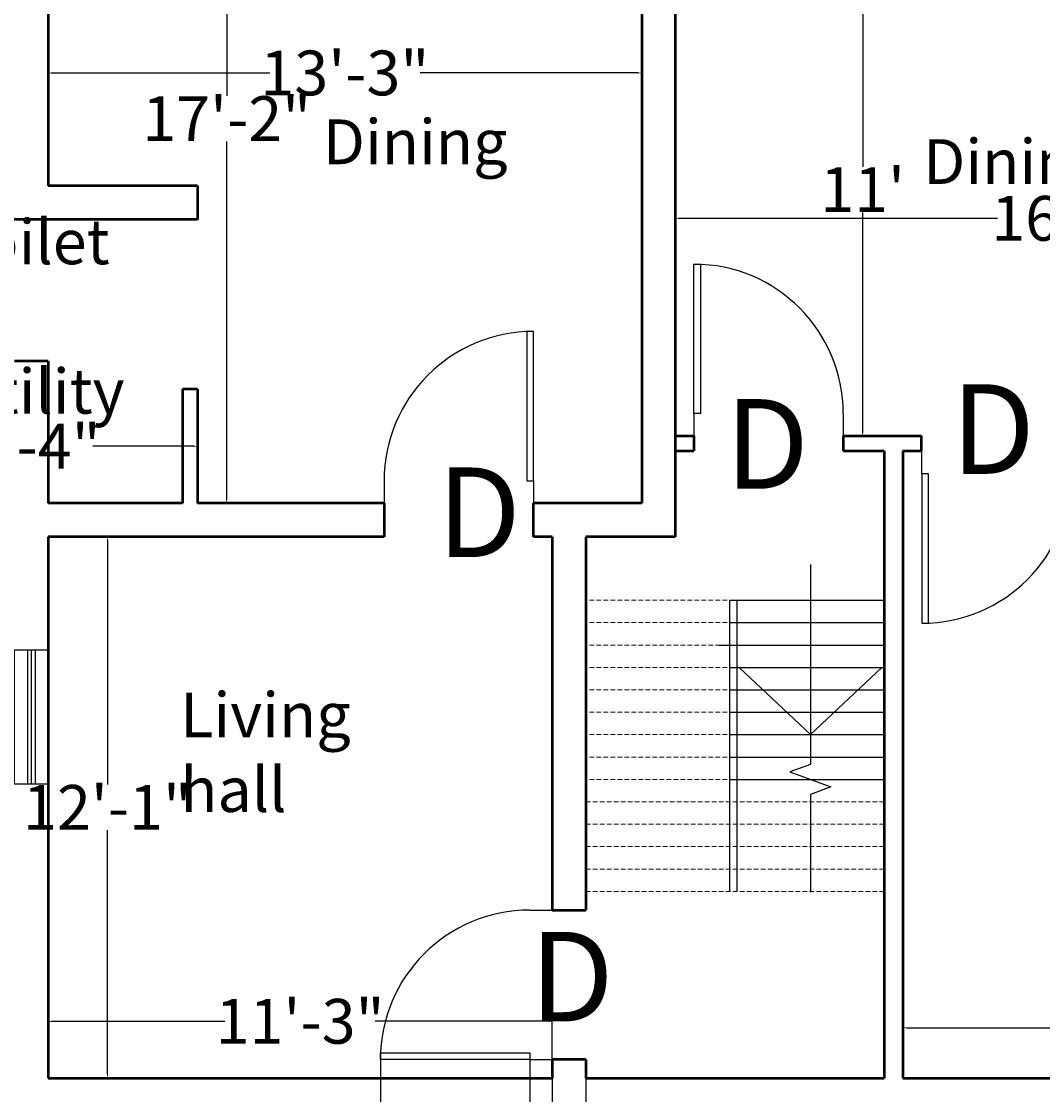
# Model space of a CAD drawing. Units: inches. Extents: x 409 to 7572, y 7 to 725.
# Tile 9 of 38: x 1698 to 1972, y 161 to 449. Entities that reach past the tile are written whole.
import ezdxf

# ---------------------------------------------------------------- set-up
doc = ezdxf.new("R2010")
doc.units = ezdxf.units.IN
doc.header["$MEASUREMENT"] = 0
doc.linetypes.add('HIDDEN', pattern=[0.375, 0.25, -0.125])
for name, color, linetype, lineweight in [('A-ANNO-DIMS', 2, 'Continuous', 18), ('A-ANNO-SYMB', 3, 'Continuous', 25), ('A-AREA-IDEN', 7, 'Continuous', 25), ('A-DOOR', 3, 'Continuous', 25), ('A-FLOR-STRS', 6, 'Continuous', 25), ('A-FLOR-STRS-OVHD', 6, 'HIDDEN', 18), ('A-GLAZ', 4, 'Continuous', 25), ('A-WALL', 7, 'Continuous', 50)]:
    doc.layers.add(name, color=color, linetype=linetype, lineweight=lineweight)
doc.styles.get("Standard").update_dxf_attribs({"font": 'arial.ttf'})
doc.dimstyles.get("Standard").update_dxf_attribs({"dimtxt": 2, "dimasz": 1, "dimexe": 0.18, "dimexo": 0.0625, "dimgap": 0.09, "dimtad": 0, "dimtih": 1, "dimtoh": 1, "dimdec": 0, "dimzin": 0, "dimdsep": 46, "dimlunit": 3, "dimtxsty": 'Standard', "dimcen": 0.09, "dimadec": 0, "dimazin": 0, "dimtfac": 1, "dimtdec": 0, "dimtofl": 0, "dimtmove": 0, "dimatfit": 3, "dimfxl": 1, "dimtolj": 1, "dimtzin": 0, "dimarcsym": 0})

# ---------------------------------------------------------------- blocks, each defined once
blk = doc.blocks.new('*U2')
for p, q in [((0, 0), (0, -6)), ((-40, 0), (-40, -6))]:
    blk.add_line(p, q)
blk.add_lwpolyline([(0, 0), (0, 40), (-1.75, 40), (-1.75, 0)], close=True)
blk.add_arc((0, 0), 40, 90, 180)
blk = doc.blocks.new('*U3')
for p, q in [((0, 0), (0, -6)), ((40, 0), (40, -6))]:
    blk.add_line(p, q)
blk.add_lwpolyline([(0, 0), (0, 40), (1.75, 40), (1.75, 0)], close=True)
blk.add_arc((0, 0), 40, 0, 90)
blk = doc.blocks.new('*U4')
for p, q in [((0, 0), (0, -6)), ((40, 0), (40, -6))]:
    blk.add_line(p, q)
blk.add_lwpolyline([(0, 0), (0, 40), (1.75, 40), (1.75, 0)], close=True)
blk.add_arc((0, 0), 40, 0, 90)
blk = doc.blocks.new('*U5')
for p, q in [((0, 0), (0, 6)), ((40, 0), (40, 6))]:
    blk.add_line(p, q)
blk.add_lwpolyline([(0, 0), (0, -40), (1.75, -40), (1.75, 0)], close=True)
blk.add_arc((0, 0), 40, 270, 0)
blk = doc.blocks.new('*D40')
at = {"layer": 'A-ANNO-DIMS', "color": 0, "lineweight": -2, "transparency": 16777216}
for p, q in [((1934.32, 165.59), (1934.32, 179.18)), ((1935.32, 179), (1982.18, 179)), ((2069.32, 179), (2022.46, 179)), ((2070.32, 165.59), (2070.32, 179.18))]:
    blk.add_line(p, q, dxfattribs=at)
at = {"layer": 'A-ANNO-DIMS', "color": 0, "transparency": 16777216}
for points in [[(1935.32, 179.16), (1935.32, 178.83), (1934.32, 179)], [(2069.32, 179.16), (2069.32, 178.83), (2070.32, 179)]]:
    blk.add_solid(points, dxfattribs=at)
at = {"layer": 'DEFPOINTS', "color": 0, "transparency": 16777216}
for p in [(2070.32, 179), (1934.32, 165.53), (2070.32, 165.53)]:
    blk.add_point(p, dxfattribs=at)
at = {"layer": 'A-ANNO-DIMS', "color": 0, "transparency": 16777216, "insert": (2002.32, 179), "char_height": 2, "attachment_point": 5}
blk.add_mtext('\\A1;{\\H6x;11\'-4"}', dxfattribs=at)
blk = doc.blocks.new('*D41')
at = {"layer": 'A-ANNO-DIMS', "color": 0, "lineweight": -2, "transparency": 16777216}
for p, q in [((1705.32, 165.59), (1705.32, 180.91)), ((1706.32, 180.73), (1752.68, 180.73)), ((1839.32, 180.73), (1792.96, 180.73)), ((1840.32, 165.59), (1840.32, 180.91))]:
    blk.add_line(p, q, dxfattribs=at)
at = {"layer": 'A-ANNO-DIMS', "color": 0, "transparency": 16777216}
for points in [[(1706.32, 180.9), (1706.32, 180.56), (1705.32, 180.73)], [(1839.32, 180.9), (1839.32, 180.56), (1840.32, 180.73)]]:
    blk.add_solid(points, dxfattribs=at)
at = {"layer": 'DEFPOINTS', "color": 0, "transparency": 16777216}
for p in [(1840.32, 180.73), (1705.32, 165.53), (1840.32, 165.53)]:
    blk.add_point(p, dxfattribs=at)
at = {"layer": 'A-ANNO-DIMS', "color": 0, "transparency": 16777216, "insert": (1772.82, 180.73), "char_height": 2, "attachment_point": 5}
blk.add_mtext('\\A1;{\\H6x;11\'-3"}', dxfattribs=at)
blk = doc.blocks.new('*D42')
at = {"layer": 'A-ANNO-DIMS', "color": 0, "lineweight": -2, "transparency": 16777216}
for p, q in [((1705.38, 310.53), (1721.42, 310.53)), ((1721.24, 309.53), (1721.24, 244.15)), ((1721.24, 166.53), (1721.24, 231.92)), ((1705.38, 165.53), (1721.42, 165.53))]:
    blk.add_line(p, q, dxfattribs=at)
at = {"layer": 'A-ANNO-DIMS', "color": 0, "transparency": 16777216}
for points in [[(1721.07, 309.53), (1721.41, 309.53), (1721.24, 310.53)], [(1721.07, 166.53), (1721.41, 166.53), (1721.24, 165.53)]]:
    blk.add_solid(points, dxfattribs=at)
at = {"layer": 'DEFPOINTS', "color": 0, "transparency": 16777216}
for p in [(1705.32, 310.53), (1705.32, 165.53), (1721.24, 165.53)]:
    blk.add_point(p, dxfattribs=at)
at = {"layer": 'A-ANNO-DIMS', "color": 0, "transparency": 16777216, "insert": (1721.24, 238.03), "char_height": 2, "attachment_point": 5}
blk.add_mtext('\\A1;{\\H6x;12\'-1"}', dxfattribs=at)
blk = doc.blocks.new('*D54')
at = {"layer": 'A-ANNO-DIMS', "color": 0, "lineweight": -2, "transparency": 16777216}
for p, q in [((1705.32, 404.59), (1705.32, 434.95)), ((1706.32, 434.77), (1764.68, 434.77)), ((1863.32, 434.77), (1804.96, 434.77)), ((1864.32, 404.59), (1864.32, 434.95))]:
    blk.add_line(p, q, dxfattribs=at)
at = {"layer": 'A-ANNO-DIMS', "color": 0, "transparency": 16777216}
for points in [[(1706.32, 434.93), (1706.32, 434.6), (1705.32, 434.77)], [(1863.32, 434.93), (1863.32, 434.6), (1864.32, 434.77)]]:
    blk.add_solid(points, dxfattribs=at)
at = {"layer": 'DEFPOINTS', "color": 0, "transparency": 16777216}
for p in [(1864.32, 434.77), (1705.32, 404.53), (1864.32, 404.53)]:
    blk.add_point(p, dxfattribs=at)
at = {"layer": 'A-ANNO-DIMS', "color": 0, "transparency": 16777216, "insert": (1784.82, 434.77), "char_height": 2, "attachment_point": 5}
blk.add_mtext('\\A1;{\\H6x;13\'-3"}', dxfattribs=at)
blk = doc.blocks.new('*D55')
at = {"layer": 'A-ANNO-DIMS', "color": 0, "lineweight": -2, "transparency": 16777216}
for p, q in [((1762.26, 525.53), (1752.98, 525.53)), ((1753.16, 524.53), (1753.16, 428.65)), ((1753.16, 320.53), (1753.16, 416.42)), ((1770.26, 319.53), (1752.98, 319.53))]:
    blk.add_line(p, q, dxfattribs=at)
at = {"layer": 'A-ANNO-DIMS', "color": 0, "transparency": 16777216}
for points in [[(1752.99, 524.53), (1753.32, 524.53), (1753.16, 525.53)], [(1752.99, 320.53), (1753.32, 320.53), (1753.16, 319.53)]]:
    blk.add_solid(points, dxfattribs=at)
at = {"layer": 'DEFPOINTS', "color": 0, "transparency": 16777216}
for p in [(1762.32, 525.53), (1753.16, 319.53), (1770.32, 319.53)]:
    blk.add_point(p, dxfattribs=at)
at = {"layer": 'A-ANNO-DIMS', "color": 0, "transparency": 16777216, "insert": (1753.16, 422.53), "char_height": 2, "attachment_point": 5}
blk.add_mtext('\\A1;{\\H6x;17\'-2"}', dxfattribs=at)
blk = doc.blocks.new('*D52')
at = {"layer": 'A-ANNO-DIMS', "color": 0, "lineweight": -2, "transparency": 16777216}
for p, q in [((1873.32, 403.47), (1873.32, 395.65)), ((2065.32, 403.47), (2065.32, 395.65)), ((1874.32, 395.83), (1959.61, 395.83)), ((2064.32, 395.83), (1979.03, 395.83))]:
    blk.add_line(p, q, dxfattribs=at)
at = {"layer": 'A-ANNO-DIMS', "color": 0, "transparency": 16777216}
for points in [[(1874.32, 396), (1874.32, 395.66), (1873.32, 395.83)], [(2064.32, 396), (2064.32, 395.66), (2065.32, 395.83)]]:
    blk.add_solid(points, dxfattribs=at)
at = {"layer": 'DEFPOINTS', "color": 0, "transparency": 16777216}
for p in [(1873.32, 403.53), (2065.32, 403.53), (2065.32, 395.83)]:
    blk.add_point(p, dxfattribs=at)
at = {"layer": 'A-ANNO-DIMS', "color": 0, "transparency": 16777216, "insert": (1969.32, 395.83), "char_height": 2, "attachment_point": 5}
blk.add_mtext("\\A1;{\\H6x;16'}", dxfattribs=at)
blk = doc.blocks.new('*D56')
at = {"layer": 'A-ANNO-DIMS', "color": 0, "lineweight": -2, "transparency": 16777216}
for p, q in [((1927.58, 469.53), (1923.34, 469.53)), ((1923.52, 468.53), (1923.52, 409.65)), ((1923.52, 338.53), (1923.52, 397.42)), ((1928.76, 337.53), (1923.34, 337.53))]:
    blk.add_line(p, q, dxfattribs=at)
at = {"layer": 'A-ANNO-DIMS', "color": 0, "transparency": 16777216}
for points in [[(1923.35, 468.53), (1923.68, 468.53), (1923.52, 469.53)], [(1923.35, 338.53), (1923.68, 338.53), (1923.52, 337.53)]]:
    blk.add_solid(points, dxfattribs=at)
at = {"layer": 'DEFPOINTS', "color": 0, "transparency": 16777216}
for p in [(1927.64, 469.53), (1923.52, 337.53), (1928.82, 337.53)]:
    blk.add_point(p, dxfattribs=at)
at = {"layer": 'A-ANNO-DIMS', "color": 0, "transparency": 16777216, "insert": (1923.52, 403.53), "char_height": 2, "attachment_point": 5}
blk.add_mtext("\\A1;{\\H6x;11'}", dxfattribs=at)
blk = doc.blocks.new('*D61')
at = {"layer": 'A-ANNO-DIMS', "color": 0, "lineweight": -2, "transparency": 16777216}
for p, q in [((1657.32, 346.33), (1657.32, 334.6)), ((1745.32, 346.33), (1745.32, 334.6)), ((1658.32, 334.78), (1685.33, 334.78)), ((1744.32, 334.78), (1717.31, 334.78))]:
    blk.add_line(p, q, dxfattribs=at)
at = {"layer": 'A-ANNO-DIMS', "color": 0, "transparency": 16777216}
for points in [[(1658.32, 334.95), (1658.32, 334.61), (1657.32, 334.78)], [(1744.32, 334.95), (1744.32, 334.61), (1745.32, 334.78)]]:
    blk.add_solid(points, dxfattribs=at)
at = {"layer": 'DEFPOINTS', "color": 0, "transparency": 16777216}
for p in [(1657.32, 346.39), (1745.32, 346.39), (1745.32, 334.78)]:
    blk.add_point(p, dxfattribs=at)
at = {"layer": 'A-ANNO-DIMS', "color": 0, "transparency": 16777216, "insert": (1701.32, 334.78), "char_height": 2, "attachment_point": 5}
blk.add_mtext('\\A1;{\\H6x;7\'-4"}', dxfattribs=at)
blk = doc.blocks.new('WIN-36')
for p, q in [((1699.82, 514.65), (1699.82, 478.65)), ((1700.82, 514.65), (1700.82, 478.65)), ((1701.82, 514.65), (1701.82, 478.65))]:
    blk.add_line(p, q)
blk.add_lwpolyline([(1705.32, 514.65), (1705.32, 478.65), (1696.32, 478.65), (1696.32, 514.65)], close=True)
blk = doc.blocks.new('*D179')
at = {"layer": 'A-ANNO-DIMS', "color": 0, "lineweight": -2, "transparency": 16777216}
for p, q in [((1840.32, 165.47), (1840.32, 118.1)), ((1849.32, 165.47), (1849.32, 118.1)), ((1841.32, 118.28), (1842.07, 118.28)), ((1848.32, 118.28), (1847.57, 118.28))]:
    blk.add_line(p, q, dxfattribs=at)
at = {"layer": 'A-ANNO-DIMS', "color": 0, "transparency": 16777216}
for points in [[(1841.32, 118.45), (1841.32, 118.11), (1840.32, 118.28)], [(1848.32, 118.45), (1848.32, 118.11), (1849.32, 118.28)]]:
    blk.add_solid(points, dxfattribs=at)
at = {"layer": 'DEFPOINTS', "color": 0, "transparency": 16777216}
for p in [(1840.32, 165.53), (1849.32, 165.53), (1849.32, 118.28)]:
    blk.add_point(p, dxfattribs=at)
at = {"layer": 'A-ANNO-DIMS', "color": 0, "transparency": 16777216, "insert": (1844.82, 118.28), "char_height": 2, "attachment_point": 5}
blk.add_mtext('\\A1;0\'-9"', dxfattribs=at)
blk = doc.blocks.new('*D182')
at = {"layer": 'A-ANNO-DIMS', "color": 0, "lineweight": -2, "transparency": 16777216}
for p, q in [((1794.32, 170.47), (1794.32, 118.1)), ((1834.32, 170.47), (1834.32, 118.1)), ((1795.32, 118.28), (1811.57, 118.28)), ((1833.32, 118.28), (1817.07, 118.28))]:
    blk.add_line(p, q, dxfattribs=at)
at = {"layer": 'A-ANNO-DIMS', "color": 0, "transparency": 16777216}
for points in [[(1795.32, 118.45), (1795.32, 118.11), (1794.32, 118.28)], [(1833.32, 118.45), (1833.32, 118.11), (1834.32, 118.28)]]:
    blk.add_solid(points, dxfattribs=at)
at = {"layer": 'DEFPOINTS', "color": 0, "transparency": 16777216}
for p in [(1794.32, 170.53), (1834.32, 170.53), (1834.32, 118.28)]:
    blk.add_point(p, dxfattribs=at)
at = {"layer": 'A-ANNO-DIMS', "color": 0, "transparency": 16777216, "insert": (1814.32, 118.28), "char_height": 2, "attachment_point": 5}
blk.add_mtext('\\A1;3\'-4"', dxfattribs=at)

msp = doc.modelspace()

# ---------------------------------------------------------------- linework, layer by layer
at = {"layer": 'A-FLOR-STRS'}
for p, q in [((1909.53, 303.06), (1909.53, 257.53)), ((1887.82, 293.53), (1929.32, 293.53)), ((1887.82, 293.53), (1887.82, 215.53)), ((1889.82, 293.53), (1889.82, 215.53)), ((1887.82, 287.53), (1929.32, 287.53)), ((1884.98, 281.53), (1929.32, 281.53)), ((1887.82, 275.53), (1929.32, 275.53)), ((1909.53, 257.53), (1890.4, 275.53)), ((1909.53, 257.53), (1928.65, 275.53)), ((1887.82, 269.53), (1929.32, 269.53)), ((1887.82, 263.53), (1929.32, 263.53)), ((1887.82, 257.53), (1929.32, 257.53)), ((1887.82, 251.53), (1929.32, 251.53)), ((1887.82, 245.53), (1929.32, 245.53))]:
    msp.add_line(p, q, dxfattribs=at)
msp.add_lwpolyline([(1909.53, 257.71), (1909.53, 249.53), (1904.03, 247.53), (1915.02, 243.53), (1909.53, 241.53), (1909.53, 215.35)], dxfattribs=at)
at = {"layer": 'A-FLOR-STRS-OVHD', "ltscale": 5}
for p, q in [((1850.32, 293.53), (1887.82, 293.53)), ((1850.32, 287.53), (1887.82, 287.53)), ((1850.32, 281.53), (1884.98, 281.53)), ((1850.32, 275.53), (1887.82, 275.53)), ((1850.32, 269.53), (1887.82, 269.53)), ((1850.32, 263.53), (1887.82, 263.53)), ((1850.32, 257.53), (1887.82, 257.53)), ((1850.32, 251.53), (1887.82, 251.53)), ((1850.32, 245.53), (1887.82, 245.53)), ((1849.32, 239.53), (1929.32, 239.53)), ((1849.32, 233.53), (1929.32, 233.53)), ((1849.32, 227.53), (1929.32, 227.53)), ((1849.32, 221.53), (1929.32, 221.53)), ((1849.32, 215.53), (1887.82, 215.53)), ((1849.32, 215.53), (1929.32, 215.53))]:
    msp.add_line(p, q, dxfattribs=at)
at = {"layer": 'A-WALL'}
for p, q in [((1705.32, 525.53), (1705.32, 404.53)), ((1864.32, 525.53), (1864.32, 319.53)), ((1873.32, 469.53), (1873.32, 337.53)), ((1745.32, 404.53), (1705.32, 404.53)), ((1745.32, 404.53), (1745.32, 395.53)), ((1705.32, 395.53), (1657.32, 395.53)), ((1745.32, 395.53), (1705.32, 395.53)), ((1705.32, 357.53), (1696.32, 357.53)), ((1705.32, 357.53), (1705.32, 319.53)), ((1741.32, 350.03), (1741.32, 319.53)), ((1745.32, 350.03), (1741.32, 350.03)), ((1745.32, 350.03), (1745.32, 319.53)), ((1873.32, 337.53), (1878.32, 337.53)), ((1873.32, 337.53), (1873.32, 333.53)), ((1878.32, 337.53), (1878.32, 333.53)), ((1918.32, 337.53), (1939.32, 337.53)), ((1918.32, 337.53), (1918.32, 333.53)), ((1939.32, 333.53), (1939.32, 337.53)), ((1873.32, 333.53), (1878.32, 333.53)), ((1873.32, 333.53), (1873.32, 310.53)), ((1918.32, 333.53), (1929.32, 333.53)), ((1929.32, 333.53), (1929.32, 165.53)), ((1934.32, 333.53), (1939.32, 333.53)), ((1934.32, 333.53), (1934.32, 165.53)), ((1741.32, 319.53), (1705.32, 319.53)), ((1795.32, 319.53), (1745.32, 319.53)), ((1795.32, 319.53), (1795.32, 310.53)), ((1864.32, 319.53), (1835.32, 319.53)), ((1835.32, 310.53), (1835.32, 319.53)), ((1795.32, 310.53), (1705.32, 310.53)), ((1705.32, 310.53), (1705.32, 165.53)), ((1840.32, 310.53), (1835.32, 310.53)), ((1840.32, 310.53), (1840.32, 210.53)), ((1873.32, 310.53), (1849.32, 310.53)), ((1849.32, 310.53), (1849.32, 210.53)), ((1840.32, 210.53), (1849.32, 210.53)), ((1840.32, 170.53), (1840.32, 165.53)), ((1849.32, 170.53), (1840.32, 170.53)), ((1849.32, 170.53), (1849.32, 165.53)), ((1705.32, 165.53), (1840.32, 165.53)), ((1849.32, 165.53), (1929.32, 165.53)), ((1934.32, 165.53), (2070.32, 165.53))]:
    msp.add_line(p, q, dxfattribs=at)

# ---------------------------------------------------------------- block references
at = {"layer": 'A-DOOR'}
for name, p in [('*U4', (1878.32, 343.53)), ('*U2', (1835.32, 325.53)), ('*U5', (1939.38, 327.37))]:
    msp.add_blockref(name, p, dxfattribs=at)
at = {"layer": 'A-DOOR', "rotation": 90}
msp.add_blockref('*U3', (1834.32, 170.53), dxfattribs=at)
at = {"layer": 'A-GLAZ'}
msp.add_blockref('WIN-36', (0, -234.38), dxfattribs=at)

# ---------------------------------------------------------------- texts
at = {"layer": 'A-ANNO-SYMB', "char_height": 24, "attachment_point": 1}
for insert in [(1947.15, 351.37), (1886.62, 347.4), (1809.46, 329.09), (1834.32, 204.69)]:
    msp.add_mtext_dynamic_manual_height_columns('D', width=19.1972, gutter_width=1, heights=[0], dxfattribs=dict(at, insert=insert))
at = {"layer": 'A-AREA-IDEN', "char_height": 12, "attachment_point": 1}
for s, width, insert in [('Dining ', 67.5069, (1778.93, 422.33)), ('Dining ', 67.5069, (1939.75, 417.03)), ('toilet / utility', 49.2946, (1681.32, 395.53)), ('Living hall', 58.8843, (1740.74, 268.81))]:
    msp.add_mtext_dynamic_manual_height_columns(s, width=width, gutter_width=1, heights=[0], dxfattribs=dict(at, insert=insert))

# ---------------------------------------------------------------- dimensions: what is measured, and where the dimension line sits
at = {"layer": 'A-ANNO-DIMS'}
dim = msp.add_linear_dim(base=(1753.16, 319.53), p1=(1762.32, 525.53), p2=(1770.32, 319.53), angle=90, text='{\\H6x;<>}', dimstyle='Standard', override={"dimclrd": 0, "dimclre": 0, "dimclrt": 0}, dxfattribs=at)
dim.commit()
dim.dimension.update_dxf_attribs({"geometry": '*D55', "text_midpoint": (1753.16, 422.53), "dimtype": 160})
for base, p1, p2, picture, middle in [((1923.52, 337.53), (1927.64, 469.53), (1928.82, 337.53), '*D56', (1923.52, 403.53)), ((1721.24, 165.53), (1705.32, 310.53), (1705.32, 165.53), '*D42', (1721.24, 238.03))]:
    dim = msp.add_linear_dim(base=base, p1=p1, p2=p2, angle=90, text='{\\H6x;<>}', dimstyle='Standard', override={"dimclrd": 0, "dimclre": 0, "dimclrt": 0}, dxfattribs=at)
    dim.commit()
    dim.dimension.update_dxf_attribs({"geometry": picture, "text_midpoint": middle})
for base, p1, p2, picture, middle in [((1864.32, 434.77), (1705.32, 404.53), (1864.32, 404.53), '*D54', (1784.82, 434.77)), ((1745.32, 334.78), (1657.32, 346.39), (1745.32, 346.39), '*D61', (1701.32, 334.78)), ((1840.32, 180.73), (1705.32, 165.53), (1840.32, 165.53), '*D41', (1772.82, 180.73)), ((2070.32, 179), (1934.32, 165.53), (2070.32, 165.53), '*D40', (2002.32, 179))]:
    dim = msp.add_linear_dim(base=base, p1=p1, p2=p2, text='{\\H6x;<>}', dimstyle='Standard', override={"dimclrd": 0, "dimclre": 0, "dimclrt": 0}, dxfattribs=at)
    dim.commit()
    dim.dimension.update_dxf_attribs({"geometry": picture, "text_midpoint": middle})
dim = msp.add_linear_dim(base=(2065.32, 395.83), p1=(1873.32, 403.53), p2=(2065.32, 403.53), text='{\\H6x;<>}', dimstyle='Standard', override={"dimclrd": 0, "dimclre": 0, "dimclrt": 0}, dxfattribs=at)
dim.commit()
dim.dimension.update_dxf_attribs({"geometry": '*D52', "text_midpoint": (1969.32, 395.83), "dimtype": 160})
for base, p1, p2, picture, middle in [((1834.32, 118.28), (1794.32, 170.53), (1834.32, 170.53), '*D182', (1814.32, 118.28)), ((1849.32, 118.28), (1840.32, 165.53), (1849.32, 165.53), '*D179', (1844.82, 118.28))]:
    dim = msp.add_linear_dim(base=base, p1=p1, p2=p2, dimstyle='Standard', override={"dimdec": 1, "dimlfac": 1, "dimrnd": 0, "dimzin": 1, "dimdsep": 46, "dimlunit": 4, "dimfrac": 2}, dxfattribs=at)
    dim.commit()
    dim.dimension.update_dxf_attribs({"geometry": picture, "text_midpoint": middle})

doc.saveas('drawing.dxf')
